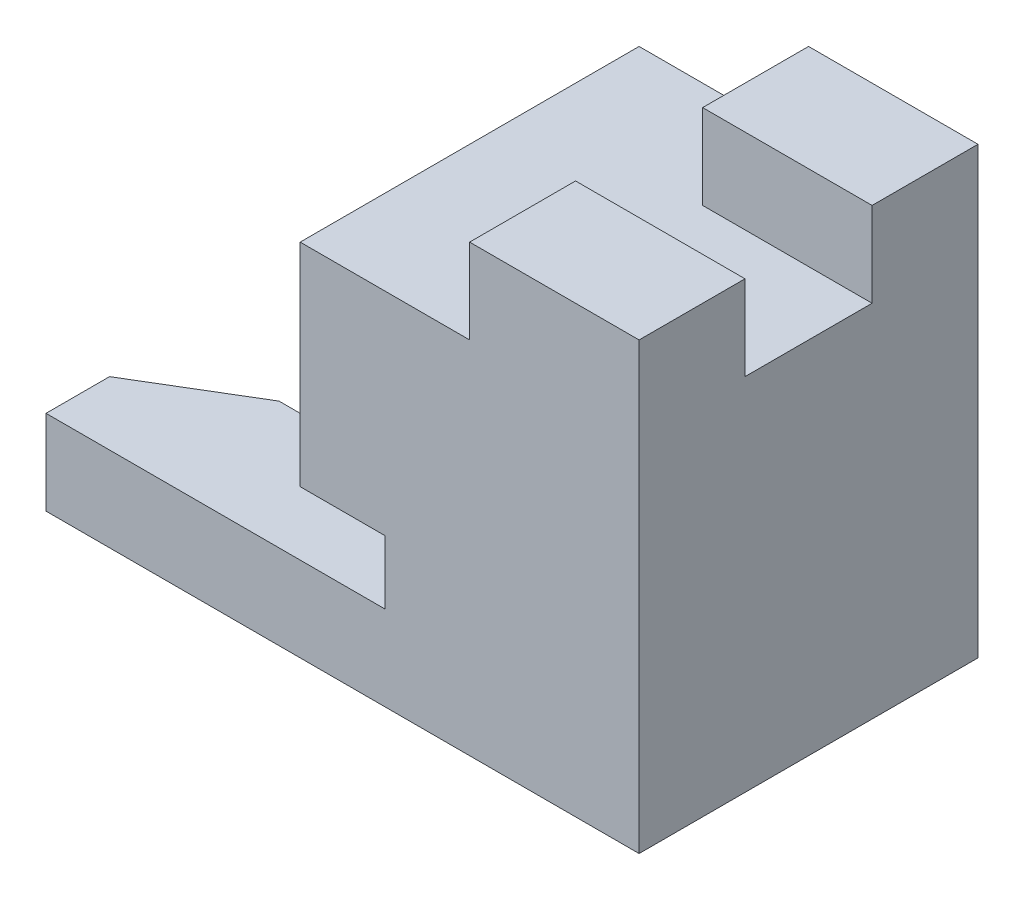
ISO-10303-21;
HEADER;
FILE_DESCRIPTION(('STEP AP214'),'2;1');
FILE_NAME('part.step','',(''),(''),'','','');
FILE_SCHEMA(('AUTOMOTIVE_DESIGN { 1 0 10303 214 1 1 1 1 }'));
ENDSEC;
DATA;
#1=APPLICATION_CONTEXT('core data for automotive mechanical design processes');
#2=APPLICATION_PROTOCOL_DEFINITION('international standard','automotive_design',2000,#1);
#3=PRODUCT_CONTEXT('',#1,'mechanical');
#4=PRODUCT('Part','Part','',(#3));
#5=PRODUCT_RELATED_PRODUCT_CATEGORY('part','',(#4));
#6=PRODUCT_DEFINITION_FORMATION('','',#4);
#7=PRODUCT_DEFINITION_CONTEXT('part definition',#1,'design');
#8=PRODUCT_DEFINITION('design','',#6,#7);
#9=PRODUCT_DEFINITION_SHAPE('','',#8);
#10=(LENGTH_UNIT() NAMED_UNIT(*) SI_UNIT(.MILLI.,.METRE.));
#11=(NAMED_UNIT(*) PLANE_ANGLE_UNIT() SI_UNIT($,.RADIAN.));
#12=(NAMED_UNIT(*) SI_UNIT($,.STERADIAN.) SOLID_ANGLE_UNIT());
#13=UNCERTAINTY_MEASURE_WITH_UNIT(LENGTH_MEASURE(1.E-05),#10,'distance_accuracy_value','');
#14=(GEOMETRIC_REPRESENTATION_CONTEXT(3) GLOBAL_UNCERTAINTY_ASSIGNED_CONTEXT((#13)) GLOBAL_UNIT_ASSIGNED_CONTEXT((#10,
#11,#12)) REPRESENTATION_CONTEXT('',''));
#15=CARTESIAN_POINT('',(0.,0.,0.));
#16=DIRECTION('',(0.,0.,1.));
#17=DIRECTION('',(1.,0.,0.));
#18=AXIS2_PLACEMENT_3D('',#15,#16,#17);
#19=CARTESIAN_POINT('',(0.,0.,80.));
#20=DIRECTION('',(1.,0.,0.));
#21=DIRECTION('',(0.,0.,-1.));
#22=AXIS2_PLACEMENT_3D('',#19,#20,#21);
#23=PLANE('',#22);
#24=DIRECTION('',(0.,-1.,0.));
#25=VECTOR('',#24,1.);
#26=CARTESIAN_POINT('',(0.,366.773517561173,65.));
#27=LINE('',#26,#25);
#28=CARTESIAN_POINT('',(0.,20.,65.));
#29=VERTEX_POINT('',#28);
#30=CARTESIAN_POINT('',(0.,0.,65.));
#31=VERTEX_POINT('',#30);
#32=EDGE_CURVE('E232',#29,#31,#27,.T.);
#33=ORIENTED_EDGE('',*,*,#32,.T.);
#34=DIRECTION('',(0.,0.,-1.));
#35=VECTOR('',#34,1.);
#36=CARTESIAN_POINT('',(0.,0.,80.));
#37=LINE('',#36,#35);
#38=CARTESIAN_POINT('',(0.,0.,80.));
#39=VERTEX_POINT('',#38);
#40=EDGE_CURVE('E11',#39,#31,#37,.T.);
#41=ORIENTED_EDGE('',*,*,#40,.F.);
#42=DIRECTION('',(0.,-1.,0.));
#43=VECTOR('',#42,1.);
#44=CARTESIAN_POINT('',(0.,0.,80.));
#45=LINE('',#44,#43);
#46=CARTESIAN_POINT('',(0.,20.,80.));
#47=VERTEX_POINT('',#46);
#48=EDGE_CURVE('E278',#47,#39,#45,.T.);
#49=ORIENTED_EDGE('',*,*,#48,.F.);
#50=DIRECTION('',(0.,0.,-1.));
#51=VECTOR('',#50,1.);
#52=CARTESIAN_POINT('',(0.,20.,80.));
#53=LINE('',#52,#51);
#54=EDGE_CURVE('E197',#47,#29,#53,.T.);
#55=ORIENTED_EDGE('',*,*,#54,.T.);
#56=EDGE_LOOP('',(#33,#41,#49,#55));
#57=FACE_BOUND('',#56,.T.);
#58=ADVANCED_FACE('F44',(#57),#23,.F.);
#59=DIRECTION('',(0.,-1.,0.));
#60=VECTOR('',#59,1.);
#61=CARTESIAN_POINT('',(0.,366.773517561173,15.));
#62=LINE('',#61,#60);
#63=CARTESIAN_POINT('',(0.,20.,15.));
#64=VERTEX_POINT('',#63);
#65=CARTESIAN_POINT('',(0.,0.,15.));
#66=VERTEX_POINT('',#65);
#67=EDGE_CURVE('E205',#64,#66,#62,.T.);
#68=ORIENTED_EDGE('',*,*,#67,.F.);
#69=CARTESIAN_POINT('',(0.,20.,0.));
#70=VERTEX_POINT('',#69);
#71=EDGE_CURVE('E183',#64,#70,#53,.T.);
#72=ORIENTED_EDGE('',*,*,#71,.T.);
#73=DIRECTION('',(0.,-1.,0.));
#74=VECTOR('',#73,1.);
#75=CARTESIAN_POINT('',(0.,0.,0.));
#76=LINE('',#75,#74);
#77=CARTESIAN_POINT('',(0.,0.,0.));
#78=VERTEX_POINT('',#77);
#79=EDGE_CURVE('E271',#70,#78,#76,.T.);
#80=ORIENTED_EDGE('',*,*,#79,.T.);
#81=EDGE_CURVE('E55',#66,#78,#37,.T.);
#82=ORIENTED_EDGE('',*,*,#81,.F.);
#83=EDGE_LOOP('',(#68,#72,#80,#82));
#84=FACE_BOUND('',#83,.T.);
#85=ADVANCED_FACE('F201',(#84),#23,.F.);
#86=CARTESIAN_POINT('',(0.,0.,80.));
#87=DIRECTION('',(0.,1.,0.));
#88=DIRECTION('',(0.,0.,1.));
#89=AXIS2_PLACEMENT_3D('',#86,#87,#88);
#90=PLANE('',#89);
#91=DIRECTION('',(0.857492925712544,0.,0.514495755427526));
#92=VECTOR('',#91,1.);
#93=CARTESIAN_POINT('',(0.,0.,15.));
#94=LINE('',#93,#92);
#95=CARTESIAN_POINT('',(25.,0.,30.));
#96=VERTEX_POINT('',#95);
#97=EDGE_CURVE('E209',#66,#96,#94,.T.);
#98=ORIENTED_EDGE('',*,*,#97,.F.);
#99=ORIENTED_EDGE('',*,*,#81,.T.);
#100=DIRECTION('',(1.,0.,0.));
#101=VECTOR('',#100,1.);
#102=CARTESIAN_POINT('',(0.,0.,0.));
#103=LINE('',#102,#101);
#104=CARTESIAN_POINT('',(140.,0.,0.));
#105=VERTEX_POINT('',#104);
#106=EDGE_CURVE('E296',#78,#105,#103,.T.);
#107=ORIENTED_EDGE('',*,*,#106,.T.);
#108=DIRECTION('',(0.,0.,-1.));
#109=VECTOR('',#108,1.);
#110=CARTESIAN_POINT('',(140.,0.,80.));
#111=LINE('',#110,#109);
#112=CARTESIAN_POINT('',(140.,0.,80.));
#113=VERTEX_POINT('',#112);
#114=EDGE_CURVE('E323',#113,#105,#111,.T.);
#115=ORIENTED_EDGE('',*,*,#114,.F.);
#116=DIRECTION('',(1.,0.,0.));
#117=VECTOR('',#116,1.);
#118=CARTESIAN_POINT('',(0.,0.,80.));
#119=LINE('',#118,#117);
#120=EDGE_CURVE('E281',#39,#113,#119,.T.);
#121=ORIENTED_EDGE('',*,*,#120,.F.);
#122=ORIENTED_EDGE('',*,*,#40,.T.);
#123=DIRECTION('',(-0.857492925712544,0.,0.514495755427526));
#124=VECTOR('',#123,1.);
#125=CARTESIAN_POINT('',(0.,0.,65.));
#126=LINE('',#125,#124);
#127=CARTESIAN_POINT('',(25.,0.,50.));
#128=VERTEX_POINT('',#127);
#129=EDGE_CURVE('E64',#128,#31,#126,.T.);
#130=ORIENTED_EDGE('',*,*,#129,.F.);
#131=DIRECTION('',(-1.,0.,0.));
#132=VECTOR('',#131,1.);
#133=CARTESIAN_POINT('',(50.,0.,50.));
#134=LINE('',#133,#132);
#135=CARTESIAN_POINT('',(50.,0.,50.));
#136=VERTEX_POINT('',#135);
#137=EDGE_CURVE('E390',#136,#128,#134,.T.);
#138=ORIENTED_EDGE('',*,*,#137,.F.);
#139=DIRECTION('',(0.,0.,1.));
#140=VECTOR('',#139,1.);
#141=CARTESIAN_POINT('',(50.,0.,40.));
#142=LINE('',#141,#140);
#143=CARTESIAN_POINT('',(50.,0.,40.));
#144=VERTEX_POINT('',#143);
#145=EDGE_CURVE('E386',#144,#136,#142,.T.);
#146=ORIENTED_EDGE('',*,*,#145,.F.);
#147=DIRECTION('',(0.,0.,1.));
#148=VECTOR('',#147,1.);
#149=CARTESIAN_POINT('',(50.,0.,40.));
#150=LINE('',#149,#148);
#151=CARTESIAN_POINT('',(50.,0.,30.));
#152=VERTEX_POINT('',#151);
#153=EDGE_CURVE('E412',#152,#144,#150,.T.);
#154=ORIENTED_EDGE('',*,*,#153,.F.);
#155=DIRECTION('',(1.,0.,0.));
#156=VECTOR('',#155,1.);
#157=CARTESIAN_POINT('',(50.,0.,30.));
#158=LINE('',#157,#156);
#159=EDGE_CURVE('E56',#96,#152,#158,.T.);
#160=ORIENTED_EDGE('',*,*,#159,.F.);
#161=EDGE_LOOP('',(#98,#99,#107,#115,#121,#122,#130,#138,#146,#154,#160));
#162=FACE_BOUND('',#161,.T.);
#163=ADVANCED_FACE('F328',(#162),#90,.F.);
#164=CARTESIAN_POINT('',(0.,20.,80.));
#165=DIRECTION('',(0.,-1.,0.));
#166=DIRECTION('',(0.,0.,-1.));
#167=AXIS2_PLACEMENT_3D('',#164,#165,#166);
#168=PLANE('',#167);
#169=DIRECTION('',(-0.857492925712544,0.,0.514495755427526));
#170=VECTOR('',#169,1.);
#171=CARTESIAN_POINT('',(0.,20.,65.));
#172=LINE('',#171,#170);
#173=CARTESIAN_POINT('',(25.,20.,50.));
#174=VERTEX_POINT('',#173);
#175=EDGE_CURVE('E391',#174,#29,#172,.T.);
#176=ORIENTED_EDGE('',*,*,#175,.T.);
#177=ORIENTED_EDGE('',*,*,#54,.F.);
#178=DIRECTION('',(-1.,0.,0.));
#179=VECTOR('',#178,1.);
#180=CARTESIAN_POINT('',(0.,20.,80.));
#181=LINE('',#180,#179);
#182=CARTESIAN_POINT('',(80.,20.,80.));
#183=VERTEX_POINT('',#182);
#184=EDGE_CURVE('E196',#183,#47,#181,.T.);
#185=ORIENTED_EDGE('',*,*,#184,.F.);
#186=DIRECTION('',(0.,0.,-1.));
#187=VECTOR('',#186,1.);
#188=CARTESIAN_POINT('',(80.,20.,80.));
#189=LINE('',#188,#187);
#190=CARTESIAN_POINT('',(80.,20.,0.));
#191=VERTEX_POINT('',#190);
#192=EDGE_CURVE('E311',#183,#191,#189,.T.);
#193=ORIENTED_EDGE('',*,*,#192,.T.);
#194=DIRECTION('',(-1.,0.,0.));
#195=VECTOR('',#194,1.);
#196=CARTESIAN_POINT('',(0.,20.,0.));
#197=LINE('',#196,#195);
#198=EDGE_CURVE('E194',#191,#70,#197,.T.);
#199=ORIENTED_EDGE('',*,*,#198,.T.);
#200=ORIENTED_EDGE('',*,*,#71,.F.);
#201=DIRECTION('',(0.857492925712544,0.,0.514495755427526));
#202=VECTOR('',#201,1.);
#203=CARTESIAN_POINT('',(0.,20.,15.));
#204=LINE('',#203,#202);
#205=CARTESIAN_POINT('',(25.,20.,30.));
#206=VERTEX_POINT('',#205);
#207=EDGE_CURVE('E187',#64,#206,#204,.T.);
#208=ORIENTED_EDGE('',*,*,#207,.T.);
#209=DIRECTION('',(1.,0.,0.));
#210=VECTOR('',#209,1.);
#211=CARTESIAN_POINT('',(50.,20.,30.));
#212=LINE('',#211,#210);
#213=CARTESIAN_POINT('',(50.,20.,30.));
#214=VERTEX_POINT('',#213);
#215=EDGE_CURVE('E211',#206,#214,#212,.T.);
#216=ORIENTED_EDGE('',*,*,#215,.T.);
#217=DIRECTION('',(0.,0.,1.));
#218=VECTOR('',#217,1.);
#219=CARTESIAN_POINT('',(50.,20.,40.));
#220=LINE('',#219,#218);
#221=CARTESIAN_POINT('',(50.,20.,40.));
#222=VERTEX_POINT('',#221);
#223=EDGE_CURVE('E212',#214,#222,#220,.T.);
#224=ORIENTED_EDGE('',*,*,#223,.T.);
#225=DIRECTION('',(0.,0.,1.));
#226=VECTOR('',#225,1.);
#227=CARTESIAN_POINT('',(50.,20.,40.));
#228=LINE('',#227,#226);
#229=CARTESIAN_POINT('',(50.,20.,50.));
#230=VERTEX_POINT('',#229);
#231=EDGE_CURVE('E399',#222,#230,#228,.T.);
#232=ORIENTED_EDGE('',*,*,#231,.T.);
#233=DIRECTION('',(-1.,0.,0.));
#234=VECTOR('',#233,1.);
#235=CARTESIAN_POINT('',(50.,20.,50.));
#236=LINE('',#235,#234);
#237=EDGE_CURVE('E394',#230,#174,#236,.T.);
#238=ORIENTED_EDGE('',*,*,#237,.T.);
#239=EDGE_LOOP('',(#176,#177,#185,#193,#199,#200,#208,#216,#224,#232,#238));
#240=FACE_BOUND('',#239,.T.);
#241=ADVANCED_FACE('F190',(#240),#168,.F.);
#242=CARTESIAN_POINT('',(100.,105.,0.));
#243=DIRECTION('',(-1.,0.,0.));
#244=DIRECTION('',(0.,0.,1.));
#245=AXIS2_PLACEMENT_3D('',#242,#243,#244);
#246=PLANE('',#245);
#247=DIRECTION('',(0.,1.,0.));
#248=VECTOR('',#247,1.);
#249=CARTESIAN_POINT('',(100.,85.,25.));
#250=LINE('',#249,#248);
#251=CARTESIAN_POINT('',(100.,85.,25.));
#252=VERTEX_POINT('',#251);
#253=CARTESIAN_POINT('',(100.,105.,25.));
#254=VERTEX_POINT('',#253);
#255=EDGE_CURVE('E247',#252,#254,#250,.T.);
#256=ORIENTED_EDGE('',*,*,#255,.T.);
#257=DIRECTION('',(0.,0.,1.));
#258=VECTOR('',#257,1.);
#259=CARTESIAN_POINT('',(100.,105.,0.));
#260=LINE('',#259,#258);
#261=CARTESIAN_POINT('',(100.,105.,0.));
#262=VERTEX_POINT('',#261);
#263=EDGE_CURVE('E272',#262,#254,#260,.T.);
#264=ORIENTED_EDGE('',*,*,#263,.F.);
#265=DIRECTION('',(0.,-1.,0.));
#266=VECTOR('',#265,1.);
#267=CARTESIAN_POINT('',(100.,105.,0.));
#268=LINE('',#267,#266);
#269=CARTESIAN_POINT('',(100.,85.,0.));
#270=VERTEX_POINT('',#269);
#271=EDGE_CURVE('E259',#262,#270,#268,.T.);
#272=ORIENTED_EDGE('',*,*,#271,.T.);
#273=DIRECTION('',(0.,0.,1.));
#274=VECTOR('',#273,1.);
#275=CARTESIAN_POINT('',(100.,85.,0.));
#276=LINE('',#275,#274);
#277=EDGE_CURVE('E268',#270,#252,#276,.T.);
#278=ORIENTED_EDGE('',*,*,#277,.T.);
#279=EDGE_LOOP('',(#256,#264,#272,#278));
#280=FACE_BOUND('',#279,.T.);
#281=ADVANCED_FACE('F341',(#280),#246,.T.);
#282=CARTESIAN_POINT('',(140.,105.,0.));
#283=DIRECTION('',(0.,1.,0.));
#284=DIRECTION('',(0.,0.,1.));
#285=AXIS2_PLACEMENT_3D('',#282,#283,#284);
#286=PLANE('',#285);
#287=DIRECTION('',(-1.,0.,0.));
#288=VECTOR('',#287,1.);
#289=CARTESIAN_POINT('',(100.,105.,25.));
#290=LINE('',#289,#288);
#291=CARTESIAN_POINT('',(140.,105.,25.));
#292=VERTEX_POINT('',#291);
#293=EDGE_CURVE('E236',#292,#254,#290,.T.);
#294=ORIENTED_EDGE('',*,*,#293,.F.);
#295=DIRECTION('',(0.,0.,1.));
#296=VECTOR('',#295,1.);
#297=CARTESIAN_POINT('',(140.,105.,0.));
#298=LINE('',#297,#296);
#299=CARTESIAN_POINT('',(140.,105.,0.));
#300=VERTEX_POINT('',#299);
#301=EDGE_CURVE('E280',#300,#292,#298,.T.);
#302=ORIENTED_EDGE('',*,*,#301,.F.);
#303=DIRECTION('',(-1.,0.,0.));
#304=VECTOR('',#303,1.);
#305=CARTESIAN_POINT('',(140.,105.,0.));
#306=LINE('',#305,#304);
#307=EDGE_CURVE('E258',#300,#262,#306,.T.);
#308=ORIENTED_EDGE('',*,*,#307,.T.);
#309=ORIENTED_EDGE('',*,*,#263,.T.);
#310=EDGE_LOOP('',(#294,#302,#308,#309));
#311=FACE_BOUND('',#310,.T.);
#312=ADVANCED_FACE('F337',(#311),#286,.T.);
#313=CARTESIAN_POINT('',(60.,85.,80.));
#314=DIRECTION('',(0.,-1.,0.));
#315=DIRECTION('',(0.,0.,-1.));
#316=AXIS2_PLACEMENT_3D('',#313,#314,#315);
#317=PLANE('',#316);
#318=ORIENTED_EDGE('',*,*,#277,.F.);
#319=DIRECTION('',(-1.,0.,0.));
#320=VECTOR('',#319,1.);
#321=CARTESIAN_POINT('',(60.,85.,0.));
#322=LINE('',#321,#320);
#323=CARTESIAN_POINT('',(60.,85.,0.));
#324=VERTEX_POINT('',#323);
#325=EDGE_CURVE('E304',#270,#324,#322,.T.);
#326=ORIENTED_EDGE('',*,*,#325,.T.);
#327=DIRECTION('',(0.,0.,-1.));
#328=VECTOR('',#327,1.);
#329=CARTESIAN_POINT('',(60.,85.,80.));
#330=LINE('',#329,#328);
#331=CARTESIAN_POINT('',(60.,85.,80.));
#332=VERTEX_POINT('',#331);
#333=EDGE_CURVE('E321',#332,#324,#330,.T.);
#334=ORIENTED_EDGE('',*,*,#333,.F.);
#335=DIRECTION('',(-1.,0.,0.));
#336=VECTOR('',#335,1.);
#337=CARTESIAN_POINT('',(60.,85.,80.));
#338=LINE('',#337,#336);
#339=CARTESIAN_POINT('',(100.,85.,80.));
#340=VERTEX_POINT('',#339);
#341=EDGE_CURVE('E289',#340,#332,#338,.T.);
#342=ORIENTED_EDGE('',*,*,#341,.F.);
#343=CARTESIAN_POINT('',(100.,85.,55.));
#344=VERTEX_POINT('',#343);
#345=EDGE_CURVE('E275',#344,#340,#276,.T.);
#346=ORIENTED_EDGE('',*,*,#345,.F.);
#347=DIRECTION('',(1.,0.,0.));
#348=VECTOR('',#347,1.);
#349=CARTESIAN_POINT('',(100.,85.,55.));
#350=LINE('',#349,#348);
#351=CARTESIAN_POINT('',(140.,85.,55.));
#352=VERTEX_POINT('',#351);
#353=EDGE_CURVE('E231',#344,#352,#350,.T.);
#354=ORIENTED_EDGE('',*,*,#353,.T.);
#355=DIRECTION('',(0.,0.,-1.));
#356=VECTOR('',#355,1.);
#357=CARTESIAN_POINT('',(140.,85.,25.));
#358=LINE('',#357,#356);
#359=CARTESIAN_POINT('',(140.,85.,25.));
#360=VERTEX_POINT('',#359);
#361=EDGE_CURVE('E240',#352,#360,#358,.T.);
#362=ORIENTED_EDGE('',*,*,#361,.T.);
#363=DIRECTION('',(-1.,0.,0.));
#364=VECTOR('',#363,1.);
#365=CARTESIAN_POINT('',(100.,85.,25.));
#366=LINE('',#365,#364);
#367=EDGE_CURVE('E238',#360,#252,#366,.T.);
#368=ORIENTED_EDGE('',*,*,#367,.T.);
#369=EDGE_LOOP('',(#318,#326,#334,#342,#346,#354,#362,#368));
#370=FACE_BOUND('',#369,.T.);
#371=ADVANCED_FACE('F350',(#370),#317,.F.);
#372=CARTESIAN_POINT('',(140.,85.,80.));
#373=DIRECTION('',(-1.,0.,0.));
#374=DIRECTION('',(0.,0.,1.));
#375=AXIS2_PLACEMENT_3D('',#372,#373,#374);
#376=PLANE('',#375);
#377=ORIENTED_EDGE('',*,*,#301,.T.);
#378=DIRECTION('',(0.,1.,0.));
#379=VECTOR('',#378,1.);
#380=CARTESIAN_POINT('',(140.,85.,25.));
#381=LINE('',#380,#379);
#382=EDGE_CURVE('E248',#360,#292,#381,.T.);
#383=ORIENTED_EDGE('',*,*,#382,.F.);
#384=ORIENTED_EDGE('',*,*,#361,.F.);
#385=DIRECTION('',(0.,1.,0.));
#386=VECTOR('',#385,1.);
#387=CARTESIAN_POINT('',(140.,85.,55.));
#388=LINE('',#387,#386);
#389=CARTESIAN_POINT('',(140.,105.,55.));
#390=VERTEX_POINT('',#389);
#391=EDGE_CURVE('E252',#352,#390,#388,.T.);
#392=ORIENTED_EDGE('',*,*,#391,.T.);
#393=CARTESIAN_POINT('',(140.,105.,80.));
#394=VERTEX_POINT('',#393);
#395=EDGE_CURVE('E263',#390,#394,#298,.T.);
#396=ORIENTED_EDGE('',*,*,#395,.T.);
#397=DIRECTION('',(0.,1.,0.));
#398=VECTOR('',#397,1.);
#399=CARTESIAN_POINT('',(140.,0.,80.));
#400=LINE('',#399,#398);
#401=EDGE_CURVE('E284',#113,#394,#400,.T.);
#402=ORIENTED_EDGE('',*,*,#401,.F.);
#403=ORIENTED_EDGE('',*,*,#114,.T.);
#404=DIRECTION('',(0.,1.,0.));
#405=VECTOR('',#404,1.);
#406=CARTESIAN_POINT('',(140.,85.,0.));
#407=LINE('',#406,#405);
#408=EDGE_CURVE('E302',#105,#300,#407,.T.);
#409=ORIENTED_EDGE('',*,*,#408,.T.);
#410=EDGE_LOOP('',(#377,#383,#384,#392,#396,#402,#403,#409));
#411=FACE_BOUND('',#410,.T.);
#412=ADVANCED_FACE('F333',(#411),#376,.F.);
#413=CARTESIAN_POINT('',(60.,35.,80.));
#414=DIRECTION('',(1.,0.,0.));
#415=DIRECTION('',(0.,0.,-1.));
#416=AXIS2_PLACEMENT_3D('',#413,#414,#415);
#417=PLANE('',#416);
#418=CARTESIAN_POINT('',(60.,60.,20.));
#419=DIRECTION('',(-1.,0.,0.));
#420=DIRECTION('',(0.,0.,1.));
#421=AXIS2_PLACEMENT_3D('',#418,#419,#420);
#422=CIRCLE('',#421,10.);
#423=CARTESIAN_POINT('',(60.,60.,30.));
#424=VERTEX_POINT('',#423);
#425=EDGE_CURVE('E423',#424,#424,#422,.T.);
#426=ORIENTED_EDGE('',*,*,#425,.F.);
#427=EDGE_LOOP('',(#426));
#428=FACE_BOUND('',#427,.T.);
#429=CARTESIAN_POINT('',(60.,60.,60.));
#430=DIRECTION('',(-1.,0.,0.));
#431=DIRECTION('',(0.,0.,1.));
#432=AXIS2_PLACEMENT_3D('',#429,#430,#431);
#433=CIRCLE('',#432,9.99999999999999);
#434=CARTESIAN_POINT('',(60.,60.,70.));
#435=VERTEX_POINT('',#434);
#436=EDGE_CURVE('E413',#435,#435,#433,.T.);
#437=ORIENTED_EDGE('',*,*,#436,.F.);
#438=EDGE_LOOP('',(#437));
#439=FACE_BOUND('',#438,.T.);
#440=DIRECTION('',(0.,-1.,0.));
#441=VECTOR('',#440,1.);
#442=CARTESIAN_POINT('',(60.,35.,0.));
#443=LINE('',#442,#441);
#444=CARTESIAN_POINT('',(60.,35.,0.));
#445=VERTEX_POINT('',#444);
#446=EDGE_CURVE('E303',#324,#445,#443,.T.);
#447=ORIENTED_EDGE('',*,*,#446,.T.);
#448=DIRECTION('',(0.,0.,-1.));
#449=VECTOR('',#448,1.);
#450=CARTESIAN_POINT('',(60.,35.,80.));
#451=LINE('',#450,#449);
#452=CARTESIAN_POINT('',(60.,35.,80.));
#453=VERTEX_POINT('',#452);
#454=EDGE_CURVE('E318',#453,#445,#451,.T.);
#455=ORIENTED_EDGE('',*,*,#454,.F.);
#456=DIRECTION('',(0.,-1.,0.));
#457=VECTOR('',#456,1.);
#458=CARTESIAN_POINT('',(60.,35.,80.));
#459=LINE('',#458,#457);
#460=EDGE_CURVE('E288',#332,#453,#459,.T.);
#461=ORIENTED_EDGE('',*,*,#460,.F.);
#462=ORIENTED_EDGE('',*,*,#333,.T.);
#463=EDGE_LOOP('',(#447,#455,#461,#462));
#464=FACE_BOUND('',#463,.T.);
#465=ADVANCED_FACE('F352',(#428,#439,#464),#417,.F.);
#466=CARTESIAN_POINT('',(80.,35.,80.));
#467=DIRECTION('',(0.,1.,0.));
#468=DIRECTION('',(0.,0.,1.));
#469=AXIS2_PLACEMENT_3D('',#466,#467,#468);
#470=PLANE('',#469);
#471=DIRECTION('',(1.,0.,0.));
#472=VECTOR('',#471,1.);
#473=CARTESIAN_POINT('',(80.,35.,0.));
#474=LINE('',#473,#472);
#475=CARTESIAN_POINT('',(80.,35.,0.));
#476=VERTEX_POINT('',#475);
#477=EDGE_CURVE('E307',#445,#476,#474,.T.);
#478=ORIENTED_EDGE('',*,*,#477,.T.);
#479=DIRECTION('',(0.,0.,-1.));
#480=VECTOR('',#479,1.);
#481=CARTESIAN_POINT('',(80.,35.,80.));
#482=LINE('',#481,#480);
#483=CARTESIAN_POINT('',(80.,35.,80.));
#484=VERTEX_POINT('',#483);
#485=EDGE_CURVE('E312',#484,#476,#482,.T.);
#486=ORIENTED_EDGE('',*,*,#485,.F.);
#487=DIRECTION('',(1.,0.,0.));
#488=VECTOR('',#487,1.);
#489=CARTESIAN_POINT('',(80.,35.,80.));
#490=LINE('',#489,#488);
#491=EDGE_CURVE('E295',#453,#484,#490,.T.);
#492=ORIENTED_EDGE('',*,*,#491,.F.);
#493=ORIENTED_EDGE('',*,*,#454,.T.);
#494=EDGE_LOOP('',(#478,#486,#492,#493));
#495=FACE_BOUND('',#494,.T.);
#496=ADVANCED_FACE('F359',(#495),#470,.F.);
#497=CARTESIAN_POINT('',(80.,20.,80.));
#498=DIRECTION('',(1.,0.,0.));
#499=DIRECTION('',(0.,0.,-1.));
#500=AXIS2_PLACEMENT_3D('',#497,#498,#499);
#501=PLANE('',#500);
#502=DIRECTION('',(0.,-1.,0.));
#503=VECTOR('',#502,1.);
#504=CARTESIAN_POINT('',(80.,20.,0.));
#505=LINE('',#504,#503);
#506=EDGE_CURVE('E310',#476,#191,#505,.T.);
#507=ORIENTED_EDGE('',*,*,#506,.T.);
#508=ORIENTED_EDGE('',*,*,#192,.F.);
#509=DIRECTION('',(0.,-1.,0.));
#510=VECTOR('',#509,1.);
#511=CARTESIAN_POINT('',(80.,20.,80.));
#512=LINE('',#511,#510);
#513=EDGE_CURVE('E294',#484,#183,#512,.T.);
#514=ORIENTED_EDGE('',*,*,#513,.F.);
#515=ORIENTED_EDGE('',*,*,#485,.T.);
#516=EDGE_LOOP('',(#507,#508,#514,#515));
#517=FACE_BOUND('',#516,.T.);
#518=ADVANCED_FACE('F483',(#517),#501,.F.);
#519=CARTESIAN_POINT('',(0.,0.,80.));
#520=DIRECTION('',(0.,0.,-1.));
#521=DIRECTION('',(-1.,0.,0.));
#522=AXIS2_PLACEMENT_3D('',#519,#520,#521);
#523=PLANE('',#522);
#524=ORIENTED_EDGE('',*,*,#48,.T.);
#525=ORIENTED_EDGE('',*,*,#120,.T.);
#526=ORIENTED_EDGE('',*,*,#401,.T.);
#527=DIRECTION('',(-1.,0.,0.));
#528=VECTOR('',#527,1.);
#529=CARTESIAN_POINT('',(140.,105.,80.));
#530=LINE('',#529,#528);
#531=CARTESIAN_POINT('',(100.,105.,80.));
#532=VERTEX_POINT('',#531);
#533=EDGE_CURVE('E246',#394,#532,#530,.T.);
#534=ORIENTED_EDGE('',*,*,#533,.T.);
#535=DIRECTION('',(0.,-1.,0.));
#536=VECTOR('',#535,1.);
#537=CARTESIAN_POINT('',(100.,105.,80.));
#538=LINE('',#537,#536);
#539=EDGE_CURVE('E257',#532,#340,#538,.T.);
#540=ORIENTED_EDGE('',*,*,#539,.T.);
#541=ORIENTED_EDGE('',*,*,#341,.T.);
#542=ORIENTED_EDGE('',*,*,#460,.T.);
#543=ORIENTED_EDGE('',*,*,#491,.T.);
#544=ORIENTED_EDGE('',*,*,#513,.T.);
#545=ORIENTED_EDGE('',*,*,#184,.T.);
#546=EDGE_LOOP('',(#524,#525,#526,#534,#540,#541,#542,#543,#544,#545));
#547=FACE_BOUND('',#546,.T.);
#548=ADVANCED_FACE('F362',(#547),#523,.F.);
#549=CARTESIAN_POINT('',(0.,0.,0.));
#550=DIRECTION('',(0.,0.,-1.));
#551=DIRECTION('',(-1.,0.,0.));
#552=AXIS2_PLACEMENT_3D('',#549,#550,#551);
#553=PLANE('',#552);
#554=ORIENTED_EDGE('',*,*,#79,.F.);
#555=ORIENTED_EDGE('',*,*,#198,.F.);
#556=ORIENTED_EDGE('',*,*,#506,.F.);
#557=ORIENTED_EDGE('',*,*,#477,.F.);
#558=ORIENTED_EDGE('',*,*,#446,.F.);
#559=ORIENTED_EDGE('',*,*,#325,.F.);
#560=ORIENTED_EDGE('',*,*,#271,.F.);
#561=ORIENTED_EDGE('',*,*,#307,.F.);
#562=ORIENTED_EDGE('',*,*,#408,.F.);
#563=ORIENTED_EDGE('',*,*,#106,.F.);
#564=EDGE_LOOP('',(#554,#555,#556,#557,#558,#559,#560,#561,#562,#563));
#565=FACE_BOUND('',#564,.T.);
#566=ADVANCED_FACE('F332',(#565),#553,.T.);
#567=DIRECTION('',(0.,1.,0.));
#568=VECTOR('',#567,1.);
#569=CARTESIAN_POINT('',(100.,85.,55.));
#570=LINE('',#569,#568);
#571=CARTESIAN_POINT('',(100.,105.,55.));
#572=VERTEX_POINT('',#571);
#573=EDGE_CURVE('E241',#344,#572,#570,.T.);
#574=ORIENTED_EDGE('',*,*,#573,.F.);
#575=ORIENTED_EDGE('',*,*,#345,.T.);
#576=ORIENTED_EDGE('',*,*,#539,.F.);
#577=EDGE_CURVE('E277',#572,#532,#260,.T.);
#578=ORIENTED_EDGE('',*,*,#577,.F.);
#579=EDGE_LOOP('',(#574,#575,#576,#578));
#580=FACE_BOUND('',#579,.T.);
#581=ADVANCED_FACE('F367',(#580),#246,.T.);
#582=DIRECTION('',(1.,0.,0.));
#583=VECTOR('',#582,1.);
#584=CARTESIAN_POINT('',(100.,105.,55.));
#585=LINE('',#584,#583);
#586=EDGE_CURVE('E234',#572,#390,#585,.T.);
#587=ORIENTED_EDGE('',*,*,#586,.F.);
#588=ORIENTED_EDGE('',*,*,#577,.T.);
#589=ORIENTED_EDGE('',*,*,#533,.F.);
#590=ORIENTED_EDGE('',*,*,#395,.F.);
#591=EDGE_LOOP('',(#587,#588,#589,#590));
#592=FACE_BOUND('',#591,.T.);
#593=ADVANCED_FACE('F380',(#592),#286,.T.);
#594=CARTESIAN_POINT('',(100.,85.,25.));
#595=DIRECTION('',(0.,0.,-1.));
#596=DIRECTION('',(-1.,0.,0.));
#597=AXIS2_PLACEMENT_3D('',#594,#595,#596);
#598=PLANE('',#597);
#599=ORIENTED_EDGE('',*,*,#293,.T.);
#600=ORIENTED_EDGE('',*,*,#255,.F.);
#601=ORIENTED_EDGE('',*,*,#367,.F.);
#602=ORIENTED_EDGE('',*,*,#382,.T.);
#603=EDGE_LOOP('',(#599,#600,#601,#602));
#604=FACE_BOUND('',#603,.T.);
#605=ADVANCED_FACE('F342',(#604),#598,.F.);
#606=CARTESIAN_POINT('',(100.,85.,55.));
#607=DIRECTION('',(0.,0.,1.));
#608=DIRECTION('',(1.,0.,0.));
#609=AXIS2_PLACEMENT_3D('',#606,#607,#608);
#610=PLANE('',#609);
#611=ORIENTED_EDGE('',*,*,#586,.T.);
#612=ORIENTED_EDGE('',*,*,#391,.F.);
#613=ORIENTED_EDGE('',*,*,#353,.F.);
#614=ORIENTED_EDGE('',*,*,#573,.T.);
#615=EDGE_LOOP('',(#611,#612,#613,#614));
#616=FACE_BOUND('',#615,.T.);
#617=ADVANCED_FACE('F372',(#616),#610,.F.);
#618=CARTESIAN_POINT('',(0.,366.773517561173,65.));
#619=DIRECTION('',(-0.514495755427526,0.,-0.857492925712544));
#620=DIRECTION('',(-0.857492925712544,0.,0.514495755427526));
#621=AXIS2_PLACEMENT_3D('',#618,#619,#620);
#622=PLANE('',#621);
#623=ORIENTED_EDGE('',*,*,#175,.F.);
#624=DIRECTION('',(0.,-1.,0.));
#625=VECTOR('',#624,1.);
#626=CARTESIAN_POINT('',(25.,366.773517561173,50.));
#627=LINE('',#626,#625);
#628=EDGE_CURVE('E226',#174,#128,#627,.T.);
#629=ORIENTED_EDGE('',*,*,#628,.T.);
#630=ORIENTED_EDGE('',*,*,#129,.T.);
#631=ORIENTED_EDGE('',*,*,#32,.F.);
#632=EDGE_LOOP('',(#623,#629,#630,#631));
#633=FACE_BOUND('',#632,.T.);
#634=ADVANCED_FACE('F384',(#633),#622,.T.);
#635=CARTESIAN_POINT('',(50.,366.773517561173,50.));
#636=DIRECTION('',(0.,0.,-1.));
#637=DIRECTION('',(-1.,0.,0.));
#638=AXIS2_PLACEMENT_3D('',#635,#636,#637);
#639=PLANE('',#638);
#640=ORIENTED_EDGE('',*,*,#237,.F.);
#641=DIRECTION('',(0.,-1.,0.));
#642=VECTOR('',#641,1.);
#643=CARTESIAN_POINT('',(50.,366.773517561173,50.));
#644=LINE('',#643,#642);
#645=EDGE_CURVE('E223',#230,#136,#644,.T.);
#646=ORIENTED_EDGE('',*,*,#645,.T.);
#647=ORIENTED_EDGE('',*,*,#137,.T.);
#648=ORIENTED_EDGE('',*,*,#628,.F.);
#649=EDGE_LOOP('',(#640,#646,#647,#648));
#650=FACE_BOUND('',#649,.T.);
#651=ADVANCED_FACE('F461',(#650),#639,.T.);
#652=CARTESIAN_POINT('',(50.,366.773517561173,40.));
#653=DIRECTION('',(-1.,0.,0.));
#654=DIRECTION('',(0.,0.,1.));
#655=AXIS2_PLACEMENT_3D('',#652,#653,#654);
#656=PLANE('',#655);
#657=ORIENTED_EDGE('',*,*,#231,.F.);
#658=DIRECTION('',(0.,-1.,0.));
#659=VECTOR('',#658,1.);
#660=CARTESIAN_POINT('',(50.,366.773517561173,40.));
#661=LINE('',#660,#659);
#662=EDGE_CURVE('E225',#222,#144,#661,.T.);
#663=ORIENTED_EDGE('',*,*,#662,.T.);
#664=ORIENTED_EDGE('',*,*,#145,.T.);
#665=ORIENTED_EDGE('',*,*,#645,.F.);
#666=EDGE_LOOP('',(#657,#663,#664,#665));
#667=FACE_BOUND('',#666,.T.);
#668=ADVANCED_FACE('F410',(#667),#656,.T.);
#669=CARTESIAN_POINT('',(50.,366.773517561173,40.));
#670=DIRECTION('',(-1.,0.,0.));
#671=DIRECTION('',(0.,0.,1.));
#672=AXIS2_PLACEMENT_3D('',#669,#670,#671);
#673=PLANE('',#672);
#674=ORIENTED_EDGE('',*,*,#223,.F.);
#675=DIRECTION('',(0.,-1.,0.));
#676=VECTOR('',#675,1.);
#677=CARTESIAN_POINT('',(50.,366.773517561173,30.));
#678=LINE('',#677,#676);
#679=EDGE_CURVE('E218',#214,#152,#678,.T.);
#680=ORIENTED_EDGE('',*,*,#679,.T.);
#681=ORIENTED_EDGE('',*,*,#153,.T.);
#682=ORIENTED_EDGE('',*,*,#662,.F.);
#683=EDGE_LOOP('',(#674,#680,#681,#682));
#684=FACE_BOUND('',#683,.T.);
#685=ADVANCED_FACE('F409',(#684),#673,.T.);
#686=CARTESIAN_POINT('',(50.,366.773517561173,30.));
#687=DIRECTION('',(0.,0.,1.));
#688=DIRECTION('',(1.,0.,0.));
#689=AXIS2_PLACEMENT_3D('',#686,#687,#688);
#690=PLANE('',#689);
#691=ORIENTED_EDGE('',*,*,#215,.F.);
#692=DIRECTION('',(0.,-1.,0.));
#693=VECTOR('',#692,1.);
#694=CARTESIAN_POINT('',(25.,366.773517561173,30.));
#695=LINE('',#694,#693);
#696=EDGE_CURVE('E202',#206,#96,#695,.T.);
#697=ORIENTED_EDGE('',*,*,#696,.T.);
#698=ORIENTED_EDGE('',*,*,#159,.T.);
#699=ORIENTED_EDGE('',*,*,#679,.F.);
#700=EDGE_LOOP('',(#691,#697,#698,#699));
#701=FACE_BOUND('',#700,.T.);
#702=ADVANCED_FACE('F455',(#701),#690,.T.);
#703=CARTESIAN_POINT('',(0.,366.773517561173,15.));
#704=DIRECTION('',(-0.514495755427526,0.,0.857492925712544));
#705=DIRECTION('',(0.857492925712544,0.,0.514495755427526));
#706=AXIS2_PLACEMENT_3D('',#703,#704,#705);
#707=PLANE('',#706);
#708=ORIENTED_EDGE('',*,*,#207,.F.);
#709=ORIENTED_EDGE('',*,*,#67,.T.);
#710=ORIENTED_EDGE('',*,*,#97,.T.);
#711=ORIENTED_EDGE('',*,*,#696,.F.);
#712=EDGE_LOOP('',(#708,#709,#710,#711));
#713=FACE_BOUND('',#712,.T.);
#714=ADVANCED_FACE('F208',(#713),#707,.T.);
#715=CARTESIAN_POINT('',(100.,60.,60.));
#716=DIRECTION('',(-1.,0.,0.));
#717=DIRECTION('',(0.,0.,1.));
#718=AXIS2_PLACEMENT_3D('',#715,#716,#717);
#719=CYLINDRICAL_SURFACE('',#718,9.99999999999999);
#720=CARTESIAN_POINT('',(100.,60.,60.));
#721=DIRECTION('',(-1.,0.,0.));
#722=DIRECTION('',(0.,0.,1.));
#723=AXIS2_PLACEMENT_3D('',#720,#721,#722);
#724=CIRCLE('',#723,9.99999999999999);
#725=CARTESIAN_POINT('',(100.,60.,70.));
#726=VERTEX_POINT('',#725);
#727=EDGE_CURVE('E416',#726,#726,#724,.T.);
#728=ORIENTED_EDGE('',*,*,#727,.F.);
#729=EDGE_LOOP('',(#728));
#730=FACE_BOUND('',#729,.T.);
#731=ORIENTED_EDGE('',*,*,#436,.T.);
#732=EDGE_LOOP('',(#731));
#733=FACE_BOUND('',#732,.T.);
#734=ADVANCED_FACE('F442',(#730,#733),#719,.F.);
#735=CARTESIAN_POINT('',(100.,60.,60.));
#736=DIRECTION('',(-1.,0.,0.));
#737=DIRECTION('',(0.,0.,1.));
#738=AXIS2_PLACEMENT_3D('',#735,#736,#737);
#739=PLANE('',#738);
#740=ORIENTED_EDGE('',*,*,#727,.T.);
#741=EDGE_LOOP('',(#740));
#742=FACE_BOUND('',#741,.T.);
#743=ADVANCED_FACE('F435',(#742),#739,.T.);
#744=CARTESIAN_POINT('',(100.,60.,20.));
#745=DIRECTION('',(-1.,0.,0.));
#746=DIRECTION('',(0.,0.,1.));
#747=AXIS2_PLACEMENT_3D('',#744,#745,#746);
#748=CYLINDRICAL_SURFACE('',#747,10.);
#749=CARTESIAN_POINT('',(100.,60.,20.));
#750=DIRECTION('',(-1.,0.,0.));
#751=DIRECTION('',(0.,0.,1.));
#752=AXIS2_PLACEMENT_3D('',#749,#750,#751);
#753=CIRCLE('',#752,10.);
#754=CARTESIAN_POINT('',(100.,60.,30.));
#755=VERTEX_POINT('',#754);
#756=EDGE_CURVE('E397',#755,#755,#753,.T.);
#757=ORIENTED_EDGE('',*,*,#756,.F.);
#758=EDGE_LOOP('',(#757));
#759=FACE_BOUND('',#758,.T.);
#760=ORIENTED_EDGE('',*,*,#425,.T.);
#761=EDGE_LOOP('',(#760));
#762=FACE_BOUND('',#761,.T.);
#763=ADVANCED_FACE('F427',(#759,#762),#748,.F.);
#764=CARTESIAN_POINT('',(100.,60.,20.));
#765=DIRECTION('',(-1.,0.,0.));
#766=DIRECTION('',(0.,0.,1.));
#767=AXIS2_PLACEMENT_3D('',#764,#765,#766);
#768=PLANE('',#767);
#769=ORIENTED_EDGE('',*,*,#756,.T.);
#770=EDGE_LOOP('',(#769));
#771=FACE_BOUND('',#770,.T.);
#772=ADVANCED_FACE('F430',(#771),#768,.T.);
#773=CLOSED_SHELL('',(#58,#85,#163,#241,#281,#312,#371,#412,#465,#496,#518,#548,#566,#581,#593,
#605,#617,#634,#651,#668,#685,#702,#714,#734,#743,#763,#772));
#774=MANIFOLD_SOLID_BREP('B2',#773);
#775=ADVANCED_BREP_SHAPE_REPRESENTATION('',(#18,#774),#14);
#776=SHAPE_DEFINITION_REPRESENTATION(#9,#775);
ENDSEC;
END-ISO-10303-21;
